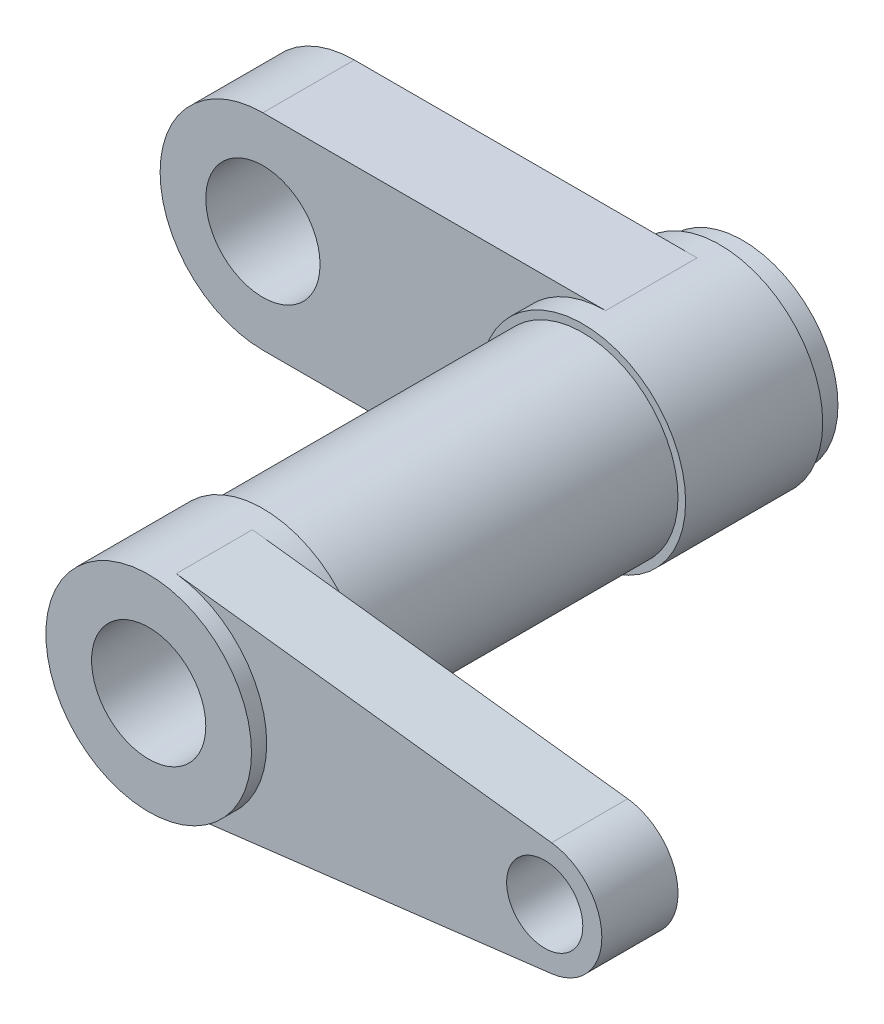
ISO-10303-21;
HEADER;
FILE_DESCRIPTION(('STEP AP214'),'2;1');
FILE_NAME('part.step','',(''),(''),'','','');
FILE_SCHEMA(('AUTOMOTIVE_DESIGN { 1 0 10303 214 1 1 1 1 }'));
ENDSEC;
DATA;
#1=APPLICATION_CONTEXT('core data for automotive mechanical design processes');
#2=APPLICATION_PROTOCOL_DEFINITION('international standard','automotive_design',2000,#1);
#3=PRODUCT_CONTEXT('',#1,'mechanical');
#4=PRODUCT('Part','Part','',(#3));
#5=PRODUCT_RELATED_PRODUCT_CATEGORY('part','',(#4));
#6=PRODUCT_DEFINITION_FORMATION('','',#4);
#7=PRODUCT_DEFINITION_CONTEXT('part definition',#1,'design');
#8=PRODUCT_DEFINITION('design','',#6,#7);
#9=PRODUCT_DEFINITION_SHAPE('','',#8);
#10=(LENGTH_UNIT() NAMED_UNIT(*) SI_UNIT(.MILLI.,.METRE.));
#11=(NAMED_UNIT(*) PLANE_ANGLE_UNIT() SI_UNIT($,.RADIAN.));
#12=(NAMED_UNIT(*) SI_UNIT($,.STERADIAN.) SOLID_ANGLE_UNIT());
#13=UNCERTAINTY_MEASURE_WITH_UNIT(LENGTH_MEASURE(1.E-05),#10,'distance_accuracy_value','');
#14=(GEOMETRIC_REPRESENTATION_CONTEXT(3) GLOBAL_UNCERTAINTY_ASSIGNED_CONTEXT((#13)) GLOBAL_UNIT_ASSIGNED_CONTEXT((#10,
#11,#12)) REPRESENTATION_CONTEXT('',''));
#15=CARTESIAN_POINT('',(0.,0.,0.));
#16=DIRECTION('',(0.,0.,1.));
#17=DIRECTION('',(1.,0.,0.));
#18=AXIS2_PLACEMENT_3D('',#15,#16,#17);
#19=CARTESIAN_POINT('',(0.,0.,51.));
#20=DIRECTION('',(0.,0.,1.));
#21=DIRECTION('',(1.,0.,0.));
#22=AXIS2_PLACEMENT_3D('',#19,#20,#21);
#23=CYLINDRICAL_SURFACE('',#22,13.5);
#24=CARTESIAN_POINT('',(0.,0.,51.));
#25=DIRECTION('',(0.,0.,1.));
#26=DIRECTION('',(1.,0.,0.));
#27=AXIS2_PLACEMENT_3D('',#24,#25,#26);
#28=CIRCLE('',#27,13.5);
#29=CARTESIAN_POINT('',(13.5,0.,51.));
#30=VERTEX_POINT('',#29);
#31=EDGE_CURVE('E150',#30,#30,#28,.T.);
#32=ORIENTED_EDGE('',*,*,#31,.T.);
#33=EDGE_LOOP('',(#32));
#34=FACE_BOUND('',#33,.T.);
#35=CARTESIAN_POINT('',(0.,0.,66.));
#36=DIRECTION('',(0.,0.,1.));
#37=DIRECTION('',(1.,0.,0.));
#38=AXIS2_PLACEMENT_3D('',#35,#36,#37);
#39=CIRCLE('',#38,13.5);
#40=CARTESIAN_POINT('',(13.5,0.,66.));
#41=VERTEX_POINT('',#40);
#42=EDGE_CURVE('E141',#41,#41,#39,.T.);
#43=ORIENTED_EDGE('',*,*,#42,.F.);
#44=EDGE_LOOP('',(#43));
#45=FACE_BOUND('',#44,.T.);
#46=DIRECTION('',(0.,0.,1.));
#47=VECTOR('',#46,1.);
#48=CARTESIAN_POINT('',(1.62,13.4024475376701,54.));
#49=LINE('',#48,#47);
#50=CARTESIAN_POINT('',(1.62,13.4024475376701,54.));
#51=VERTEX_POINT('',#50);
#52=CARTESIAN_POINT('',(1.62,13.4024475376701,64.));
#53=VERTEX_POINT('',#52);
#54=EDGE_CURVE('E63',#51,#53,#49,.T.);
#55=ORIENTED_EDGE('',*,*,#54,.F.);
#56=CARTESIAN_POINT('',(0.,0.,54.));
#57=DIRECTION('',(0.,0.,-1.));
#58=DIRECTION('',(1.,0.,0.));
#59=AXIS2_PLACEMENT_3D('',#56,#57,#58);
#60=CIRCLE('',#59,13.5);
#61=CARTESIAN_POINT('',(1.62,-13.4024475376701,54.));
#62=VERTEX_POINT('',#61);
#63=EDGE_CURVE('E57',#51,#62,#60,.T.);
#64=ORIENTED_EDGE('',*,*,#63,.T.);
#65=DIRECTION('',(0.,0.,1.));
#66=VECTOR('',#65,1.);
#67=CARTESIAN_POINT('',(1.62,-13.4024475376701,54.));
#68=LINE('',#67,#66);
#69=CARTESIAN_POINT('',(1.62,-13.4024475376701,64.));
#70=VERTEX_POINT('',#69);
#71=EDGE_CURVE('E145',#62,#70,#68,.T.);
#72=ORIENTED_EDGE('',*,*,#71,.T.);
#73=CARTESIAN_POINT('',(0.,0.,64.));
#74=DIRECTION('',(0.,0.,-1.));
#75=DIRECTION('',(1.,0.,0.));
#76=AXIS2_PLACEMENT_3D('',#73,#74,#75);
#77=CIRCLE('',#76,13.5);
#78=EDGE_CURVE('E126',#53,#70,#77,.T.);
#79=ORIENTED_EDGE('',*,*,#78,.F.);
#80=EDGE_LOOP('',(#55,#64,#72,#79));
#81=FACE_BOUND('',#80,.T.);
#82=ADVANCED_FACE('F41',(#34,#45,#81),#23,.T.);
#83=CARTESIAN_POINT('',(0.,0.,66.));
#84=DIRECTION('',(0.,0.,-1.));
#85=DIRECTION('',(-1.,0.,0.));
#86=AXIS2_PLACEMENT_3D('',#83,#84,#85);
#87=CYLINDRICAL_SURFACE('',#86,12.5);
#88=CARTESIAN_POINT('',(0.,0.,9.));
#89=DIRECTION('',(0.,0.,1.));
#90=DIRECTION('',(1.,0.,0.));
#91=AXIS2_PLACEMENT_3D('',#88,#89,#90);
#92=CIRCLE('',#91,12.5);
#93=CARTESIAN_POINT('',(12.5,0.,9.));
#94=VERTEX_POINT('',#93);
#95=EDGE_CURVE('E196',#94,#94,#92,.F.);
#96=ORIENTED_EDGE('',*,*,#95,.F.);
#97=EDGE_LOOP('',(#96));
#98=FACE_BOUND('',#97,.T.);
#99=CARTESIAN_POINT('',(0.,0.,51.));
#100=DIRECTION('',(0.,0.,1.));
#101=DIRECTION('',(1.,0.,0.));
#102=AXIS2_PLACEMENT_3D('',#99,#100,#101);
#103=CIRCLE('',#102,12.5);
#104=CARTESIAN_POINT('',(12.5,0.,51.));
#105=VERTEX_POINT('',#104);
#106=EDGE_CURVE('E11',#105,#105,#103,.T.);
#107=ORIENTED_EDGE('',*,*,#106,.F.);
#108=EDGE_LOOP('',(#107));
#109=FACE_BOUND('',#108,.T.);
#110=ADVANCED_FACE('F225',(#98,#109),#87,.T.);
#111=CARTESIAN_POINT('',(0.,0.,9.));
#112=DIRECTION('',(0.,0.,1.));
#113=DIRECTION('',(1.,0.,0.));
#114=AXIS2_PLACEMENT_3D('',#111,#112,#113);
#115=PLANE('',#114);
#116=CARTESIAN_POINT('',(0.,0.,9.));
#117=DIRECTION('',(0.,0.,1.));
#118=DIRECTION('',(1.,0.,0.));
#119=AXIS2_PLACEMENT_3D('',#116,#117,#118);
#120=CIRCLE('',#119,13.5);
#121=CARTESIAN_POINT('',(13.5,0.,9.));
#122=VERTEX_POINT('',#121);
#123=EDGE_CURVE('E205',#122,#122,#120,.T.);
#124=ORIENTED_EDGE('',*,*,#123,.T.);
#125=EDGE_LOOP('',(#124));
#126=FACE_BOUND('',#125,.T.);
#127=ORIENTED_EDGE('',*,*,#95,.T.);
#128=EDGE_LOOP('',(#127));
#129=FACE_BOUND('',#128,.T.);
#130=ADVANCED_FACE('F212',(#126,#129),#115,.T.);
#131=CARTESIAN_POINT('',(0.,0.,-9.));
#132=DIRECTION('',(0.,0.,1.));
#133=DIRECTION('',(1.,0.,0.));
#134=AXIS2_PLACEMENT_3D('',#131,#132,#133);
#135=PLANE('',#134);
#136=CARTESIAN_POINT('',(0.,0.,-9.));
#137=DIRECTION('',(0.,0.,1.));
#138=DIRECTION('',(1.,0.,0.));
#139=AXIS2_PLACEMENT_3D('',#136,#137,#138);
#140=CIRCLE('',#139,13.5);
#141=CARTESIAN_POINT('',(13.5,0.,-9.));
#142=VERTEX_POINT('',#141);
#143=EDGE_CURVE('E203',#142,#142,#140,.T.);
#144=ORIENTED_EDGE('',*,*,#143,.F.);
#145=EDGE_LOOP('',(#144));
#146=FACE_BOUND('',#145,.T.);
#147=CARTESIAN_POINT('',(0.,0.,-8.99999999999999));
#148=DIRECTION('',(0.,0.,1.));
#149=DIRECTION('',(1.,0.,0.));
#150=AXIS2_PLACEMENT_3D('',#147,#148,#149);
#151=CIRCLE('',#150,12.5);
#152=CARTESIAN_POINT('',(12.5,0.,-8.99999999999999));
#153=VERTEX_POINT('',#152);
#154=EDGE_CURVE('E47',#153,#153,#151,.F.);
#155=ORIENTED_EDGE('',*,*,#154,.F.);
#156=EDGE_LOOP('',(#155));
#157=FACE_BOUND('',#156,.T.);
#158=ADVANCED_FACE('F211',(#146,#157),#135,.F.);
#159=CARTESIAN_POINT('',(0.,0.,9.));
#160=DIRECTION('',(0.,0.,-1.));
#161=DIRECTION('',(-1.,0.,0.));
#162=AXIS2_PLACEMENT_3D('',#159,#160,#161);
#163=CYLINDRICAL_SURFACE('',#162,13.5);
#164=DIRECTION('',(0.,0.,-1.));
#165=VECTOR('',#164,1.);
#166=CARTESIAN_POINT('',(0.,13.5,6.));
#167=LINE('',#166,#165);
#168=CARTESIAN_POINT('',(0.,13.5,6.));
#169=VERTEX_POINT('',#168);
#170=CARTESIAN_POINT('',(0.,13.5,-6.));
#171=VERTEX_POINT('',#170);
#172=EDGE_CURVE('E184',#169,#171,#167,.T.);
#173=ORIENTED_EDGE('',*,*,#172,.F.);
#174=CARTESIAN_POINT('',(0.,0.,6.));
#175=DIRECTION('',(0.,0.,1.));
#176=DIRECTION('',(1.,0.,0.));
#177=AXIS2_PLACEMENT_3D('',#174,#175,#176);
#178=CIRCLE('',#177,13.5);
#179=CARTESIAN_POINT('',(0.,-13.5,6.));
#180=VERTEX_POINT('',#179);
#181=EDGE_CURVE('E156',#169,#180,#178,.T.);
#182=ORIENTED_EDGE('',*,*,#181,.T.);
#183=DIRECTION('',(0.,0.,-1.));
#184=VECTOR('',#183,1.);
#185=CARTESIAN_POINT('',(0.,-13.5,6.));
#186=LINE('',#185,#184);
#187=CARTESIAN_POINT('',(0.,-13.5,-6.));
#188=VERTEX_POINT('',#187);
#189=EDGE_CURVE('E189',#180,#188,#186,.T.);
#190=ORIENTED_EDGE('',*,*,#189,.T.);
#191=CARTESIAN_POINT('',(0.,0.,-6.));
#192=DIRECTION('',(0.,0.,1.));
#193=DIRECTION('',(1.,0.,0.));
#194=AXIS2_PLACEMENT_3D('',#191,#192,#193);
#195=CIRCLE('',#194,13.5);
#196=EDGE_CURVE('E168',#171,#188,#195,.T.);
#197=ORIENTED_EDGE('',*,*,#196,.F.);
#198=EDGE_LOOP('',(#173,#182,#190,#197));
#199=FACE_BOUND('',#198,.T.);
#200=ORIENTED_EDGE('',*,*,#123,.F.);
#201=EDGE_LOOP('',(#200));
#202=FACE_BOUND('',#201,.T.);
#203=ORIENTED_EDGE('',*,*,#143,.T.);
#204=EDGE_LOOP('',(#203));
#205=FACE_BOUND('',#204,.T.);
#206=ADVANCED_FACE('F213',(#199,#202,#205),#163,.T.);
#207=CARTESIAN_POINT('',(0.,0.,-12.));
#208=DIRECTION('',(0.,0.,1.));
#209=DIRECTION('',(1.,0.,0.));
#210=AXIS2_PLACEMENT_3D('',#207,#208,#209);
#211=CIRCLE('',#210,12.5);
#212=CARTESIAN_POINT('',(12.5,0.,-12.));
#213=VERTEX_POINT('',#212);
#214=EDGE_CURVE('E195',#213,#213,#211,.T.);
#215=ORIENTED_EDGE('',*,*,#214,.T.);
#216=EDGE_LOOP('',(#215));
#217=FACE_BOUND('',#216,.T.);
#218=ORIENTED_EDGE('',*,*,#154,.T.);
#219=EDGE_LOOP('',(#218));
#220=FACE_BOUND('',#219,.T.);
#221=ADVANCED_FACE('F207',(#217,#220),#87,.T.);
#222=CARTESIAN_POINT('',(0.,0.,-12.));
#223=DIRECTION('',(0.,0.,1.));
#224=DIRECTION('',(1.,0.,0.));
#225=AXIS2_PLACEMENT_3D('',#222,#223,#224);
#226=PLANE('',#225);
#227=CARTESIAN_POINT('',(0.,0.,-12.));
#228=DIRECTION('',(0.,0.,1.));
#229=DIRECTION('',(1.,0.,0.));
#230=AXIS2_PLACEMENT_3D('',#227,#228,#229);
#231=CIRCLE('',#230,7.5);
#232=CARTESIAN_POINT('',(7.5,0.,-12.));
#233=VERTEX_POINT('',#232);
#234=EDGE_CURVE('E190',#233,#233,#231,.T.);
#235=ORIENTED_EDGE('',*,*,#234,.T.);
#236=EDGE_LOOP('',(#235));
#237=FACE_BOUND('',#236,.T.);
#238=ORIENTED_EDGE('',*,*,#214,.F.);
#239=EDGE_LOOP('',(#238));
#240=FACE_BOUND('',#239,.T.);
#241=ADVANCED_FACE('F266',(#237,#240),#226,.F.);
#242=CARTESIAN_POINT('',(0.,0.,9.));
#243=DIRECTION('',(0.,0.,-1.));
#244=DIRECTION('',(-1.,0.,0.));
#245=AXIS2_PLACEMENT_3D('',#242,#243,#244);
#246=CYLINDRICAL_SURFACE('',#245,7.5);
#247=CARTESIAN_POINT('',(0.,0.,66.));
#248=DIRECTION('',(0.,0.,1.));
#249=DIRECTION('',(1.,0.,0.));
#250=AXIS2_PLACEMENT_3D('',#247,#248,#249);
#251=CIRCLE('',#250,7.5);
#252=CARTESIAN_POINT('',(7.5,0.,66.));
#253=VERTEX_POINT('',#252);
#254=EDGE_CURVE('E191',#253,#253,#251,.T.);
#255=ORIENTED_EDGE('',*,*,#254,.T.);
#256=EDGE_LOOP('',(#255));
#257=FACE_BOUND('',#256,.T.);
#258=ORIENTED_EDGE('',*,*,#234,.F.);
#259=EDGE_LOOP('',(#258));
#260=FACE_BOUND('',#259,.T.);
#261=ADVANCED_FACE('F43',(#257,#260),#246,.F.);
#262=CARTESIAN_POINT('',(0.,0.,66.));
#263=DIRECTION('',(0.,0.,1.));
#264=DIRECTION('',(1.,0.,0.));
#265=AXIS2_PLACEMENT_3D('',#262,#263,#264);
#266=PLANE('',#265);
#267=ORIENTED_EDGE('',*,*,#254,.F.);
#268=EDGE_LOOP('',(#267));
#269=FACE_BOUND('',#268,.T.);
#270=ORIENTED_EDGE('',*,*,#42,.T.);
#271=EDGE_LOOP('',(#270));
#272=FACE_BOUND('',#271,.T.);
#273=ADVANCED_FACE('F262',(#269,#272),#266,.T.);
#274=CARTESIAN_POINT('',(0.,-13.5,6.));
#275=DIRECTION('',(0.,1.,0.));
#276=DIRECTION('',(0.,0.,1.));
#277=AXIS2_PLACEMENT_3D('',#274,#275,#276);
#278=PLANE('',#277);
#279=DIRECTION('',(1.,0.,0.));
#280=VECTOR('',#279,1.);
#281=CARTESIAN_POINT('',(0.,-13.5,-6.));
#282=LINE('',#281,#280);
#283=CARTESIAN_POINT('',(-45.,-13.5,-6.));
#284=VERTEX_POINT('',#283);
#285=EDGE_CURVE('E147',#284,#188,#282,.T.);
#286=ORIENTED_EDGE('',*,*,#285,.T.);
#287=ORIENTED_EDGE('',*,*,#189,.F.);
#288=DIRECTION('',(1.,0.,0.));
#289=VECTOR('',#288,1.);
#290=CARTESIAN_POINT('',(0.,-13.5,6.));
#291=LINE('',#290,#289);
#292=CARTESIAN_POINT('',(-45.,-13.5,6.));
#293=VERTEX_POINT('',#292);
#294=EDGE_CURVE('E153',#293,#180,#291,.T.);
#295=ORIENTED_EDGE('',*,*,#294,.F.);
#296=DIRECTION('',(0.,0.,-1.));
#297=VECTOR('',#296,1.);
#298=CARTESIAN_POINT('',(-45.,-13.5,6.));
#299=LINE('',#298,#297);
#300=EDGE_CURVE('E170',#293,#284,#299,.T.);
#301=ORIENTED_EDGE('',*,*,#300,.T.);
#302=EDGE_LOOP('',(#286,#287,#295,#301));
#303=FACE_BOUND('',#302,.T.);
#304=ADVANCED_FACE('F257',(#303),#278,.F.);
#305=CARTESIAN_POINT('',(0.,13.5,6.));
#306=DIRECTION('',(0.,1.,0.));
#307=DIRECTION('',(0.,0.,1.));
#308=AXIS2_PLACEMENT_3D('',#305,#306,#307);
#309=PLANE('',#308);
#310=DIRECTION('',(1.,0.,0.));
#311=VECTOR('',#310,1.);
#312=CARTESIAN_POINT('',(0.,13.5,-6.));
#313=LINE('',#312,#311);
#314=CARTESIAN_POINT('',(-45.,13.5,-6.));
#315=VERTEX_POINT('',#314);
#316=EDGE_CURVE('E172',#315,#171,#313,.T.);
#317=ORIENTED_EDGE('',*,*,#316,.F.);
#318=DIRECTION('',(0.,0.,-1.));
#319=VECTOR('',#318,1.);
#320=CARTESIAN_POINT('',(-45.,13.5,6.));
#321=LINE('',#320,#319);
#322=CARTESIAN_POINT('',(-45.,13.5,6.));
#323=VERTEX_POINT('',#322);
#324=EDGE_CURVE('E185',#323,#315,#321,.T.);
#325=ORIENTED_EDGE('',*,*,#324,.F.);
#326=DIRECTION('',(1.,0.,0.));
#327=VECTOR('',#326,1.);
#328=CARTESIAN_POINT('',(0.,13.5,6.));
#329=LINE('',#328,#327);
#330=EDGE_CURVE('E157',#323,#169,#329,.T.);
#331=ORIENTED_EDGE('',*,*,#330,.T.);
#332=ORIENTED_EDGE('',*,*,#172,.T.);
#333=EDGE_LOOP('',(#317,#325,#331,#332));
#334=FACE_BOUND('',#333,.T.);
#335=ADVANCED_FACE('F258',(#334),#309,.T.);
#336=CARTESIAN_POINT('',(-45.,0.,6.));
#337=DIRECTION('',(0.,0.,-1.));
#338=DIRECTION('',(-1.,0.,0.));
#339=AXIS2_PLACEMENT_3D('',#336,#337,#338);
#340=CYLINDRICAL_SURFACE('',#339,13.5);
#341=CARTESIAN_POINT('',(-45.,0.,-6.));
#342=DIRECTION('',(0.,0.,1.));
#343=DIRECTION('',(1.,0.,0.));
#344=AXIS2_PLACEMENT_3D('',#341,#342,#343);
#345=CIRCLE('',#344,13.5);
#346=EDGE_CURVE('E177',#315,#284,#345,.T.);
#347=ORIENTED_EDGE('',*,*,#346,.T.);
#348=ORIENTED_EDGE('',*,*,#300,.F.);
#349=CARTESIAN_POINT('',(-45.,0.,6.));
#350=DIRECTION('',(0.,0.,1.));
#351=DIRECTION('',(1.,0.,0.));
#352=AXIS2_PLACEMENT_3D('',#349,#350,#351);
#353=CIRCLE('',#352,13.5);
#354=EDGE_CURVE('E165',#323,#293,#353,.T.);
#355=ORIENTED_EDGE('',*,*,#354,.F.);
#356=ORIENTED_EDGE('',*,*,#324,.T.);
#357=EDGE_LOOP('',(#347,#348,#355,#356));
#358=FACE_BOUND('',#357,.T.);
#359=ADVANCED_FACE('F252',(#358),#340,.T.);
#360=CARTESIAN_POINT('',(-45.,0.,6.));
#361=DIRECTION('',(0.,0.,-1.));
#362=DIRECTION('',(-1.,0.,0.));
#363=AXIS2_PLACEMENT_3D('',#360,#361,#362);
#364=CYLINDRICAL_SURFACE('',#363,7.5);
#365=CARTESIAN_POINT('',(-45.,0.,6.));
#366=DIRECTION('',(0.,0.,1.));
#367=DIRECTION('',(1.,0.,0.));
#368=AXIS2_PLACEMENT_3D('',#365,#366,#367);
#369=CIRCLE('',#368,7.5);
#370=CARTESIAN_POINT('',(-37.5,0.,6.));
#371=VERTEX_POINT('',#370);
#372=EDGE_CURVE('E163',#371,#371,#369,.T.);
#373=ORIENTED_EDGE('',*,*,#372,.T.);
#374=EDGE_LOOP('',(#373));
#375=FACE_BOUND('',#374,.T.);
#376=CARTESIAN_POINT('',(-45.,0.,-6.));
#377=DIRECTION('',(0.,0.,1.));
#378=DIRECTION('',(1.,0.,0.));
#379=AXIS2_PLACEMENT_3D('',#376,#377,#378);
#380=CIRCLE('',#379,7.5);
#381=CARTESIAN_POINT('',(-37.5,0.,-6.));
#382=VERTEX_POINT('',#381);
#383=EDGE_CURVE('E160',#382,#382,#380,.T.);
#384=ORIENTED_EDGE('',*,*,#383,.F.);
#385=EDGE_LOOP('',(#384));
#386=FACE_BOUND('',#385,.T.);
#387=ADVANCED_FACE('F241',(#375,#386),#364,.F.);
#388=CARTESIAN_POINT('',(0.,0.,6.));
#389=DIRECTION('',(0.,0.,1.));
#390=DIRECTION('',(1.,0.,0.));
#391=AXIS2_PLACEMENT_3D('',#388,#389,#390);
#392=PLANE('',#391);
#393=ORIENTED_EDGE('',*,*,#294,.T.);
#394=ORIENTED_EDGE('',*,*,#181,.F.);
#395=ORIENTED_EDGE('',*,*,#330,.F.);
#396=ORIENTED_EDGE('',*,*,#354,.T.);
#397=EDGE_LOOP('',(#393,#394,#395,#396));
#398=FACE_BOUND('',#397,.T.);
#399=ORIENTED_EDGE('',*,*,#372,.F.);
#400=EDGE_LOOP('',(#399));
#401=FACE_BOUND('',#400,.T.);
#402=ADVANCED_FACE('F243',(#398,#401),#392,.T.);
#403=CARTESIAN_POINT('',(0.,0.,-6.));
#404=DIRECTION('',(0.,0.,1.));
#405=DIRECTION('',(1.,0.,0.));
#406=AXIS2_PLACEMENT_3D('',#403,#404,#405);
#407=PLANE('',#406);
#408=ORIENTED_EDGE('',*,*,#285,.F.);
#409=ORIENTED_EDGE('',*,*,#346,.F.);
#410=ORIENTED_EDGE('',*,*,#316,.T.);
#411=ORIENTED_EDGE('',*,*,#196,.T.);
#412=EDGE_LOOP('',(#408,#409,#410,#411));
#413=FACE_BOUND('',#412,.T.);
#414=ORIENTED_EDGE('',*,*,#383,.T.);
#415=EDGE_LOOP('',(#414));
#416=FACE_BOUND('',#415,.T.);
#417=ADVANCED_FACE('F245',(#413,#416),#407,.F.);
#418=CARTESIAN_POINT('',(0.,0.,51.));
#419=DIRECTION('',(0.,0.,1.));
#420=DIRECTION('',(1.,0.,0.));
#421=AXIS2_PLACEMENT_3D('',#418,#419,#420);
#422=PLANE('',#421);
#423=ORIENTED_EDGE('',*,*,#106,.T.);
#424=EDGE_LOOP('',(#423));
#425=FACE_BOUND('',#424,.T.);
#426=ORIENTED_EDGE('',*,*,#31,.F.);
#427=EDGE_LOOP('',(#426));
#428=FACE_BOUND('',#427,.T.);
#429=ADVANCED_FACE('F239',(#425,#428),#422,.F.);
#430=CARTESIAN_POINT('',(50.,0.,54.));
#431=DIRECTION('',(0.,0.,1.));
#432=DIRECTION('',(1.,0.,0.));
#433=AXIS2_PLACEMENT_3D('',#430,#431,#432);
#434=CYLINDRICAL_SURFACE('',#433,7.5);
#435=CARTESIAN_POINT('',(50.,0.,64.));
#436=DIRECTION('',(0.,0.,1.));
#437=DIRECTION('',(1.,0.,0.));
#438=AXIS2_PLACEMENT_3D('',#435,#436,#437);
#439=CIRCLE('',#438,7.5);
#440=CARTESIAN_POINT('',(50.9,-7.44580418759451,64.));
#441=VERTEX_POINT('',#440);
#442=CARTESIAN_POINT('',(50.9,7.44580418759451,64.));
#443=VERTEX_POINT('',#442);
#444=EDGE_CURVE('E137',#441,#443,#439,.T.);
#445=ORIENTED_EDGE('',*,*,#444,.F.);
#446=DIRECTION('',(0.,0.,1.));
#447=VECTOR('',#446,1.);
#448=CARTESIAN_POINT('',(50.9,-7.44580418759451,54.));
#449=LINE('',#448,#447);
#450=CARTESIAN_POINT('',(50.9,-7.44580418759451,54.));
#451=VERTEX_POINT('',#450);
#452=EDGE_CURVE('E124',#451,#441,#449,.T.);
#453=ORIENTED_EDGE('',*,*,#452,.F.);
#454=CARTESIAN_POINT('',(50.,0.,54.));
#455=DIRECTION('',(0.,0.,1.));
#456=DIRECTION('',(1.,0.,0.));
#457=AXIS2_PLACEMENT_3D('',#454,#455,#456);
#458=CIRCLE('',#457,7.5);
#459=CARTESIAN_POINT('',(50.9,7.44580418759451,54.));
#460=VERTEX_POINT('',#459);
#461=EDGE_CURVE('E116',#451,#460,#458,.T.);
#462=ORIENTED_EDGE('',*,*,#461,.T.);
#463=DIRECTION('',(0.,0.,1.));
#464=VECTOR('',#463,1.);
#465=CARTESIAN_POINT('',(50.9,7.44580418759451,54.));
#466=LINE('',#465,#464);
#467=EDGE_CURVE('E102',#460,#443,#466,.T.);
#468=ORIENTED_EDGE('',*,*,#467,.T.);
#469=EDGE_LOOP('',(#445,#453,#462,#468));
#470=FACE_BOUND('',#469,.T.);
#471=ADVANCED_FACE('F123',(#470),#434,.T.);
#472=CARTESIAN_POINT('',(1.62,-13.4024475376701,54.));
#473=DIRECTION('',(0.12,-0.992773891679269,0.));
#474=DIRECTION('',(0.992773891679269,0.12,0.));
#475=AXIS2_PLACEMENT_3D('',#472,#473,#474);
#476=PLANE('',#475);
#477=DIRECTION('',(0.992773891679268,0.12,0.));
#478=VECTOR('',#477,1.);
#479=CARTESIAN_POINT('',(1.62,-13.4024475376701,64.));
#480=LINE('',#479,#478);
#481=EDGE_CURVE('E121',#70,#441,#480,.T.);
#482=ORIENTED_EDGE('',*,*,#481,.F.);
#483=ORIENTED_EDGE('',*,*,#71,.F.);
#484=DIRECTION('',(0.992773891679268,0.12,0.));
#485=VECTOR('',#484,1.);
#486=CARTESIAN_POINT('',(1.62,-13.4024475376701,54.));
#487=LINE('',#486,#485);
#488=EDGE_CURVE('E111',#62,#451,#487,.T.);
#489=ORIENTED_EDGE('',*,*,#488,.T.);
#490=ORIENTED_EDGE('',*,*,#452,.T.);
#491=EDGE_LOOP('',(#482,#483,#489,#490));
#492=FACE_BOUND('',#491,.T.);
#493=ADVANCED_FACE('F356',(#492),#476,.T.);
#494=CARTESIAN_POINT('',(1.62,13.4024475376701,54.));
#495=DIRECTION('',(0.12,0.992773891679269,0.));
#496=DIRECTION('',(-0.992773891679269,0.12,0.));
#497=AXIS2_PLACEMENT_3D('',#494,#495,#496);
#498=PLANE('',#497);
#499=DIRECTION('',(-0.992773891679268,0.12,0.));
#500=VECTOR('',#499,1.);
#501=CARTESIAN_POINT('',(1.62,13.4024475376701,64.));
#502=LINE('',#501,#500);
#503=EDGE_CURVE('E108',#443,#53,#502,.T.);
#504=ORIENTED_EDGE('',*,*,#503,.F.);
#505=ORIENTED_EDGE('',*,*,#467,.F.);
#506=DIRECTION('',(-0.992773891679268,0.12,0.));
#507=VECTOR('',#506,1.);
#508=CARTESIAN_POINT('',(1.62,13.4024475376701,54.));
#509=LINE('',#508,#507);
#510=EDGE_CURVE('E110',#460,#51,#509,.T.);
#511=ORIENTED_EDGE('',*,*,#510,.T.);
#512=ORIENTED_EDGE('',*,*,#54,.T.);
#513=EDGE_LOOP('',(#504,#505,#511,#512));
#514=FACE_BOUND('',#513,.T.);
#515=ADVANCED_FACE('F106',(#514),#498,.T.);
#516=CARTESIAN_POINT('',(50.,0.,54.));
#517=DIRECTION('',(0.,0.,1.));
#518=DIRECTION('',(1.,0.,0.));
#519=AXIS2_PLACEMENT_3D('',#516,#517,#518);
#520=PLANE('',#519);
#521=CARTESIAN_POINT('',(50.,0.,54.));
#522=DIRECTION('',(0.,0.,1.));
#523=DIRECTION('',(1.,0.,0.));
#524=AXIS2_PLACEMENT_3D('',#521,#522,#523);
#525=CIRCLE('',#524,5.);
#526=CARTESIAN_POINT('',(55.,0.,54.));
#527=VERTEX_POINT('',#526);
#528=EDGE_CURVE('E138',#527,#527,#525,.T.);
#529=ORIENTED_EDGE('',*,*,#528,.T.);
#530=EDGE_LOOP('',(#529));
#531=FACE_BOUND('',#530,.T.);
#532=ORIENTED_EDGE('',*,*,#461,.F.);
#533=ORIENTED_EDGE('',*,*,#488,.F.);
#534=ORIENTED_EDGE('',*,*,#63,.F.);
#535=ORIENTED_EDGE('',*,*,#510,.F.);
#536=EDGE_LOOP('',(#532,#533,#534,#535));
#537=FACE_BOUND('',#536,.T.);
#538=ADVANCED_FACE('F117',(#531,#537),#520,.F.);
#539=CARTESIAN_POINT('',(50.,0.,64.));
#540=DIRECTION('',(0.,0.,1.));
#541=DIRECTION('',(1.,0.,0.));
#542=AXIS2_PLACEMENT_3D('',#539,#540,#541);
#543=PLANE('',#542);
#544=CARTESIAN_POINT('',(50.,0.,64.));
#545=DIRECTION('',(0.,0.,1.));
#546=DIRECTION('',(1.,0.,0.));
#547=AXIS2_PLACEMENT_3D('',#544,#545,#546);
#548=CIRCLE('',#547,5.);
#549=CARTESIAN_POINT('',(55.,0.,64.));
#550=VERTEX_POINT('',#549);
#551=EDGE_CURVE('E133',#550,#550,#548,.T.);
#552=ORIENTED_EDGE('',*,*,#551,.F.);
#553=EDGE_LOOP('',(#552));
#554=FACE_BOUND('',#553,.T.);
#555=ORIENTED_EDGE('',*,*,#444,.T.);
#556=ORIENTED_EDGE('',*,*,#503,.T.);
#557=ORIENTED_EDGE('',*,*,#78,.T.);
#558=ORIENTED_EDGE('',*,*,#481,.T.);
#559=EDGE_LOOP('',(#555,#556,#557,#558));
#560=FACE_BOUND('',#559,.T.);
#561=ADVANCED_FACE('F384',(#554,#560),#543,.T.);
#562=CARTESIAN_POINT('',(50.,0.,54.));
#563=DIRECTION('',(0.,0.,1.));
#564=DIRECTION('',(1.,0.,0.));
#565=AXIS2_PLACEMENT_3D('',#562,#563,#564);
#566=CYLINDRICAL_SURFACE('',#565,5.);
#567=ORIENTED_EDGE('',*,*,#528,.F.);
#568=EDGE_LOOP('',(#567));
#569=FACE_BOUND('',#568,.T.);
#570=ORIENTED_EDGE('',*,*,#551,.T.);
#571=EDGE_LOOP('',(#570));
#572=FACE_BOUND('',#571,.T.);
#573=ADVANCED_FACE('F391',(#569,#572),#566,.F.);
#574=CLOSED_SHELL('',(#82,#110,#130,#158,#206,#221,#241,#261,#273,#304,#335,#359,#387,#402,#417,
#429,#471,#493,#515,#538,#561,#573));
#575=MANIFOLD_SOLID_BREP('B2',#574);
#576=ADVANCED_BREP_SHAPE_REPRESENTATION('',(#18,#575),#14);
#577=SHAPE_DEFINITION_REPRESENTATION(#9,#576);
ENDSEC;
END-ISO-10303-21;
